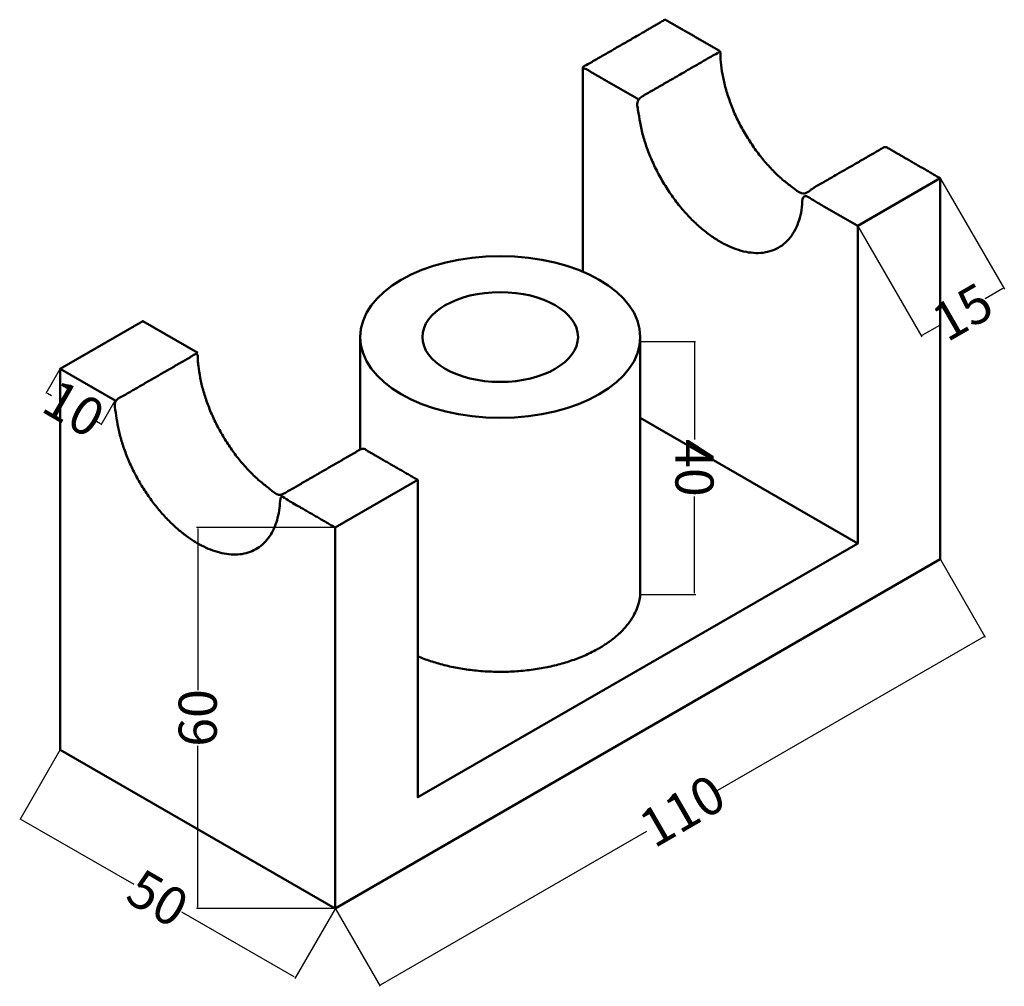
# Model space of a CAD drawing. Units: millimetres. Extents: x -6 to 149, y 15 to 167.
import ezdxf

# ---------------------------------------------------------------- set-up
doc = ezdxf.new("R2010")
doc.units = ezdxf.units.MM
doc.header["$MEASUREMENT"] = 0
doc.layers.add('M-DIMS', color=2, linetype='Continuous', lineweight=25)
doc.layers.add('M-OUTL', color=7, linetype='Continuous', lineweight=50)
doc.styles.get("Standard").update_dxf_attribs({"font": 'arial.ttf'})
doc.dimstyles.get("Standard").update_dxf_attribs({"dimtxt": 6, "dimasz": 0.18, "dimexe": 0.18, "dimexo": 0.0625, "dimgap": 0.09, "dimtad": 0, "dimtoh": 1, "dimdec": 0, "dimzin": 0, "dimdsep": 46, "dimtxsty": 'Standard', "dimcen": 0.09, "dimadec": 0, "dimazin": 0, "dimtfac": 1, "dimtdec": 0, "dimtofl": 0, "dimtmove": 0, "dimatfit": 3, "dimfxl": 1, "dimtolj": 1, "dimtzin": 0, "dimarcsym": 0})

# ---------------------------------------------------------------- blocks, each defined once
blk = doc.blocks.new('*D1')
at = {"layer": 'Defpoints', "color": 0, "transparency": 16777216}
for p in [(139.25, 82.5), (146.24, 70.39), (43.99, 27.5)]:
    blk.add_point(p, dxfattribs=at)
at = {"layer": 'M-DIMS', "color": 0, "lineweight": -2, "transparency": 16777216}
for p, q in [((139.28, 82.44), (146.33, 70.23)), ((146.09, 70.3), (104.18, 46.1)), ((51.14, 15.48), (93.05, 39.68)), ((44.02, 27.44), (51.07, 15.23))]:
    blk.add_line(p, q, dxfattribs=at)
at = {"layer": 'M-DIMS', "color": 0, "transparency": 16777216}
for points in [[(146.07, 70.32), (146.1, 70.27), (146.24, 70.39)], [(51.12, 15.5), (51.15, 15.45), (50.98, 15.39)]]:
    blk.add_solid(points, dxfattribs=at)
at = {"layer": 'M-DIMS', "color": 0, "transparency": 16777216, "insert": (98.61, 42.89), "char_height": 6, "attachment_point": 5, "rotation": 30}
blk.add_mtext('\\A1;110', dxfattribs=at)
blk = doc.blocks.new('*D2')
at = {"layer": 'Defpoints', "color": 0, "transparency": 16777216}
for p in [(91.98, 116.81), (91.99, 76.95), (100.56, 76.95)]:
    blk.add_point(p, dxfattribs=at)
at = {"layer": 'M-DIMS', "color": 0, "lineweight": -2, "transparency": 16777216}
for p, q in [((92.05, 116.81), (100.73, 116.82)), ((100.55, 116.64), (100.55, 101.38)), ((100.56, 77.13), (100.56, 92.38)), ((92.06, 76.95), (100.74, 76.95))]:
    blk.add_line(p, q, dxfattribs=at)
at = {"layer": 'M-DIMS', "color": 0, "transparency": 16777216}
for points in [[(100.58, 116.64), (100.52, 116.64), (100.55, 116.82)], [(100.59, 77.13), (100.53, 77.13), (100.56, 76.95)]]:
    blk.add_solid(points, dxfattribs=at)
at = {"layer": 'M-DIMS', "color": 0, "transparency": 16777216, "insert": (100.55, 96.88), "char_height": 6, "attachment_point": 5, "rotation": 270.016}
blk.add_mtext('\\A1;40', dxfattribs=at)
blk = doc.blocks.new('*D3')
at = {"layer": 'Defpoints', "color": 0, "transparency": 16777216}
for p in [(0.69, 52.5), (43.99, 27.5), (37.71, 16.62)]:
    blk.add_point(p, dxfattribs=at)
at = {"layer": 'M-DIMS', "color": 0, "lineweight": -2, "transparency": 16777216}
for p, q in [((0.66, 52.44), (-5.68, 41.47)), ((-5.44, 41.53), (12.27, 31.31)), ((37.55, 16.71), (19.85, 26.93)), ((43.96, 27.44), (37.62, 16.47))]:
    blk.add_line(p, q, dxfattribs=at)
at = {"layer": 'M-DIMS', "color": 0, "transparency": 16777216}
for points in [[(-5.42, 41.56), (-5.45, 41.51), (-5.59, 41.62)], [(37.57, 16.74), (37.54, 16.69), (37.71, 16.62)]]:
    blk.add_solid(points, dxfattribs=at)
at = {"layer": 'M-DIMS', "color": 0, "transparency": 16777216, "insert": (16.06, 29.12), "char_height": 6, "attachment_point": 5, "rotation": 330}
blk.add_mtext('\\A1;50', dxfattribs=at)
blk = doc.blocks.new('*D4')
at = {"layer": 'Defpoints', "color": 0, "transparency": 16777216}
for p in [(0.69, 112.5), (9.35, 107.5), (7.18, 103.75)]:
    blk.add_point(p, dxfattribs=at)
at = {"layer": 'M-DIMS', "color": 0, "lineweight": -2, "transparency": 16777216}
for p, q in [((0.66, 112.44), (-1.57, 108.59)), ((-1.32, 108.66), (-0.69, 108.3)), ((9.32, 107.44), (7.09, 103.59)), ((7.03, 103.84), (6.4, 104.2))]:
    blk.add_line(p, q, dxfattribs=at)
at = {"layer": 'M-DIMS', "color": 0, "transparency": 16777216}
for points in [[(-1.31, 108.68), (-1.34, 108.63), (-1.48, 108.75)], [(7.04, 103.86), (7.01, 103.81), (7.18, 103.75)]]:
    blk.add_solid(points, dxfattribs=at)
at = {"layer": 'M-DIMS', "color": 0, "transparency": 16777216, "insert": (2.85, 106.25), "char_height": 6, "attachment_point": 5, "rotation": 330}
blk.add_mtext('\\A1;10', dxfattribs=at)
blk = doc.blocks.new('*D5')
at = {"layer": 'Defpoints', "color": 0, "transparency": 16777216}
for p in [(139.25, 142.5), (126.26, 135), (149.24, 125.21)]:
    blk.add_point(p, dxfattribs=at)
at = {"layer": 'M-DIMS', "color": 0, "lineweight": -2, "transparency": 16777216}
for p, q in [((139.28, 142.44), (149.33, 125.05)), ((126.29, 134.94), (136.33, 117.55)), ((149.08, 125.12), (146.31, 123.52)), ((136.4, 117.8), (139.17, 119.39))]:
    blk.add_line(p, q, dxfattribs=at)
at = {"layer": 'M-DIMS', "color": 0, "transparency": 16777216}
for points in [[(149.06, 125.14), (149.09, 125.09), (149.24, 125.21)], [(136.39, 117.82), (136.42, 117.77), (136.24, 117.71)]]:
    blk.add_solid(points, dxfattribs=at)
at = {"layer": 'M-DIMS', "color": 0, "transparency": 16777216, "insert": (142.74, 121.46), "char_height": 6, "attachment_point": 5, "rotation": 30}
blk.add_mtext('\\A1;15', dxfattribs=at)
blk = doc.blocks.new('*D6')
at = {"layer": 'Defpoints', "color": 0, "transparency": 16777216}
for p in [(43.99, 87.5), (22.34, 27.5), (43.99, 27.5)]:
    blk.add_point(p, dxfattribs=at)
at = {"layer": 'M-DIMS', "color": 0, "lineweight": -2, "transparency": 16777216}
for p, q in [((43.93, 87.5), (22.16, 87.5)), ((22.34, 87.32), (22.34, 61.89)), ((22.34, 27.68), (22.34, 53.1)), ((43.93, 27.5), (22.16, 27.5))]:
    blk.add_line(p, q, dxfattribs=at)
at = {"layer": 'M-DIMS', "color": 0, "transparency": 16777216}
for points in [[(22.31, 87.32), (22.37, 87.32), (22.34, 87.5)], [(22.31, 27.68), (22.37, 27.68), (22.34, 27.5)]]:
    blk.add_solid(points, dxfattribs=at)
at = {"layer": 'M-DIMS', "color": 0, "transparency": 16777216, "insert": (22.34, 57.5), "char_height": 6, "attachment_point": 5, "rotation": 90}
blk.add_mtext('\\A1;60', dxfattribs=at)

msp = doc.modelspace()

# ---------------------------------------------------------------- linework, layer by layer
at = {"layer": 'M-OUTL'}
for p, q in [((82.96, 127.78), (82.96, 160)), ((47.92, 117.5), (47.92, 99.77))]:
    msp.add_line(p, q, dxfattribs=at)
for points in [[(0.69, 112.5), (0.69, 62.5), (0.69, 52.5), (43.99, 27.5), (139.25, 82.5), (139.25, 92.5), (139.25, 142.5), (126.26, 135), (126.26, 85), (92.02, 104.77)], [(9.35, 107.5), (0.69, 112.5), (13.68, 120), (22.34, 115)], [(43.99, 27.5), (43.99, 37.5), (43.99, 87.5), (56.98, 95), (56.98, 45), (126.26, 85)]]:
    msp.add_lwpolyline(points, dxfattribs=at)
msp.add_lwpolyline([(0.69, 62.5), (0.69, 62.5)], close=True, dxfattribs=at)
for major_axis in [(-22.05, 0), (-12.25, 0)]:
    msp.add_ellipse((69.97, 117.5), major_axis=major_axis, ratio=0.57735, dxfattribs=at)
for points, weights, knots in [([(91.62, 155), (87.29, 157.5), (82.96, 160), (89.46, 163.75), (95.95, 167.5), (100.28, 165), (104.61, 162.5), (98.12, 158.75), (91.62, 155), (91.62, 140), (104.61, 132.5), (117.6, 125), (117.6, 140), (121.93, 137.5), (126.26, 135)], [1, 1, 1, 1, 1, 1, 1, 1, 1, 0.707106781187, 1, 0.707106781187, 1, 1, 1], [0, 0, 0, 1, 1, 2, 2, 3, 3, 4, 4, 5.570796, 5.570796, 7.141593, 7.141593, 8.141593, 8.141593, 8.141593]), ([(104.61, 162.5), (104.61, 147.5), (117.6, 140), (124.1, 143.75), (130.59, 147.5), (134.92, 145), (139.25, 142.5)], [1, 0.707106781187, 1, 1, 1, 1, 1], [0, 0, 0, 1.570796, 1.570796, 2.570796, 2.570796, 3.570796, 3.570796, 3.570796]), ([(56.98, 67.21), (67.91, 62.61), (79.96, 66.15), (92.02, 69.69), (92.02, 77.5), (92.02, 97.5), (92.02, 117.5)], [1, 0.852402507188, 1, 0.852402507188, 1, 1, 1], [0, 0, 0, 1.100467, 1.100467, 2.200934, 2.200934, 3.200934, 3.200934, 3.200934]), ([(43.99, 87.5), (39.66, 90), (35.33, 92.5), (35.33, 77.5), (22.34, 85), (9.35, 92.5), (9.35, 107.5), (15.84, 111.25), (22.34, 115), (22.34, 100), (35.33, 92.5), (41.82, 96.25), (48.32, 100), (52.65, 97.5), (56.98, 95)], [1, 1, 1, 0.707106781187, 1, 0.707106781187, 1, 1, 1, 0.707106781187, 1, 1, 1, 1, 1], [0, 0, 0, 1, 1, 2.570796, 2.570796, 4.141593, 4.141593, 5.141593, 5.141593, 6.712389, 6.712389, 7.712389, 7.712389, 8.712389, 8.712389, 8.712389])]:
    msp.add_rational_spline(points, weights, degree=2, knots=knots, dxfattribs=at)

# ---------------------------------------------------------------- dimensions: what is measured, and where the dimension line sits
at = {"layer": 'M-DIMS'}
for p1, p2, distance, picture, middle in [((126.26, 135), (139.25, 142.5), -19.97, '*D5', (142.74, 121.46)), ((91.98, 116.81), (91.99, 76.95), 8.57, '*D2', (100.55, 96.88)), ((0.69, 112.5), (9.35, 107.5), -4.33, '*D4', (2.85, 106.25)), ((43.99, 87.5), (43.99, 27.5), -21.65, '*D6', (22.34, 57.5)), ((43.99, 27.5), (139.25, 82.5), -13.98, '*D1', (98.61, 42.89)), ((0.69, 52.5), (43.99, 27.5), -12.56, '*D3', (16.06, 29.12))]:
    dim = msp.add_aligned_dim(p1=p1, p2=p2, distance=distance, dimstyle='Standard', override={"dimclrd": 0, "dimclre": 0, "dimclrt": 0}, dxfattribs=at)
    dim.commit()
    dim.dimension.update_dxf_attribs({"geometry": picture, "text_midpoint": middle})

doc.saveas('drawing.dxf')
